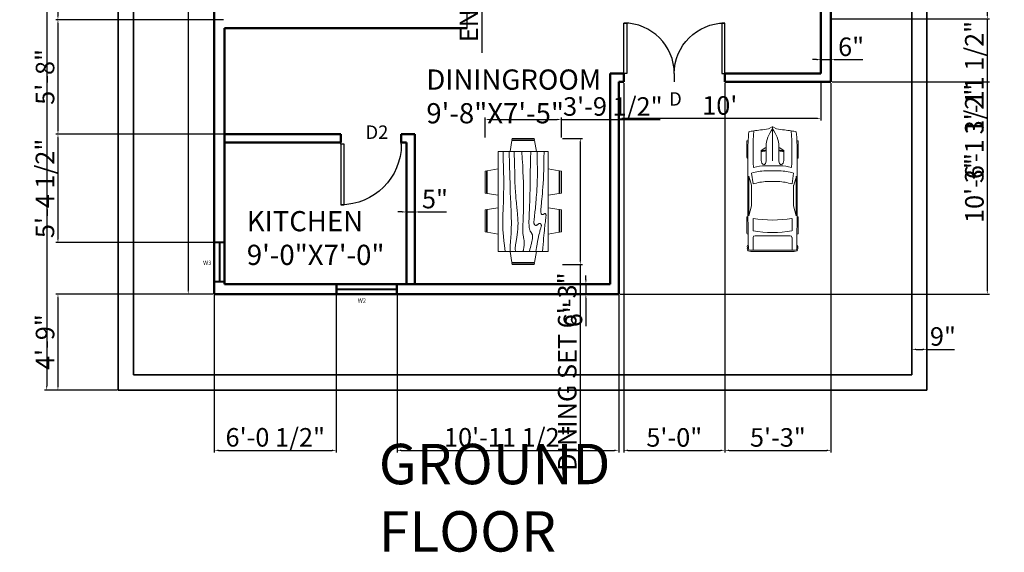
# Model space of a CAD drawing. Units: inches. Extents: x 2299 to 4423, y 1066 to 1805.
# Tile 1 of 7: x 2299 to 2884, y 1075 to 1391. Entities that reach past the tile are written whole.
import ezdxf

# ---------------------------------------------------------------- set-up
doc = ezdxf.new("R2010")
doc.units = ezdxf.units.IN
for name, color, linetype, lineweight in [('A-ANNO-DIMS', 2, 'Continuous', 18), ('A-ANNO-TEXT', 1, 'Continuous', 25), ('A-AREA-IDEN', 1, 'Continuous', 25), ('A-DOOR', 5, 'Continuous', 25), ('A-FLOR-STRS', 6, 'Continuous', 25), ('A-FURN', 8, 'Continuous', 18), ('A-GLAZ', 3, 'Continuous', 25), ('A-WALL', 7, 'Continuous', 50), ('C-PROP', 7, 'Continuous', 35)]:
    doc.layers.add(name, color=color, linetype=linetype, lineweight=lineweight)
doc.styles.get("Standard").update_dxf_attribs({"font": 'arial.ttf'})
doc.dimstyles.new('ISO-25', dxfattribs={"dimtxt": 11, "dimasz": 2.5, "dimexe": 1.25, "dimexo": 0.625, "dimtad": 1, "dimlunit": 4, "dimtxsty": 'Standard', "dimcen": 2.5, "dimadec": 0, "dimazin": 0, "dimtfac": 1, "dimtmove": 0, "dimatfit": 3, "dimfxl": 1, "dimarcsym": 0})

# ---------------------------------------------------------------- blocks, each defined once
blk = doc.blocks.new('*U2')
for p, q in [((0, 0), (0, -5)), ((30, 0), (30, -5))]:
    blk.add_line(p, q)
blk.add_lwpolyline([(0, 0), (0, 30), (1.75, 30), (1.75, 0)], close=True)
blk.add_arc((0, 0), 30, 0, 90)
blk = doc.blocks.new('Dining Set - 36 x 72 in.')
for p, q in [((-22.2343, 26.00059), (-23.4847, 17.99762)), ((-22.2304, 26), (-5.7608, 26)), ((-22, 27.5), (-22.1562, 26.50042)), ((-5.8416, 26.5), (-22.1534, 26.5)), ((-22, 27.5), (-6, 27.5)), ((-5.8437, 26.49966), (-6, 27.5)), ((-4.5152, 17.99762), (-5.7655, 25.99926)), ((5.7657, 26.00059), (4.5153, 17.99762)), ((5.7696, 26), (22.2392, 26)), ((6, 27.5), (5.8438, 26.50042)), ((22.1584, 26.5), (5.8466, 26.5)), ((6, 27.5), (22, 27.5)), ((22.1563, 26.49966), (22, 27.5)), ((23.4848, 17.99762), (22.2345, 25.99926)), ((36, 18), (-36, 18)), ((-36, 18), (-36, -18)), ((36, -18), (36, 18)), ((-45.5, 8), (-44.5004, 8.15617)), ((-45.5, 8), (-45.5, -8)), ((-44.5, -8.15843), (-44.5, 8.15338)), ((-44.0006, 8.23428), (-35.9976, 9.48474)), ((-44, 8.23041), (-44, -8.23915)), ((44.0006, 8.23428), (35.9976, 9.48474)), ((44, 8.23041), (44, -8.23915)), ((44.5, -8.15843), (44.5, 8.15338)), ((45.5, 8), (44.5005, 8.15617)), ((45.5, 8), (45.5, -8)), ((-44.4997, -8.15631), (-45.5, -8)), ((-35.9976, -9.48476), (-43.9993, -8.2345)), ((35.9976, -9.48476), (43.9993, -8.2345)), ((44.4997, -8.15631), (45.5, -8)), ((-36, -18), (36, -18)), ((-22.2343, -26.0006), (-23.4847, -17.99762)), ((-4.5152, -17.99762), (-5.7655, -25.99928)), ((5.7657, -26.0006), (4.5153, -17.99762)), ((23.4848, -17.99762), (22.2345, -25.99928)), ((-22.2304, -26), (-5.7608, -26)), ((-22, -27.5), (-22.1562, -26.50044)), ((-5.8416, -26.5), (-22.1534, -26.5)), ((-22, -27.5), (-6, -27.5)), ((-5.8437, -26.49967), (-6, -27.5)), ((5.7696, -26), (22.2392, -26)), ((6, -27.5), (5.8438, -26.50044)), ((22.1584, -26.5), (5.8466, -26.5)), ((6, -27.5), (22, -27.5)), ((22.1563, -26.49967), (22, -27.5))]:
    blk.add_line(p, q)
for points in [[(-36, 15), (-31.1772, 14.97754), (-26.8079, 14.91406), (-22.8538, 14.81543), (-19.276, 14.6875), (-16.0362, 14.53613), (-13.0957, 14.36718), (-10.4159, 14.18652), (-7.9583, 14), (-5.6904, 13.81315), (-3.6035, 13.63021), (-1.6954, 13.45508), (0.0365, 13.29166), (1.5945, 13.14388), (2.9811, 13.01562), (4.1988, 12.9108), (5.25, 12.83333), (6.1393, 12.78613), (6.8802, 12.76823), (7.4883, 12.77767), (7.9792, 12.8125), (8.3685, 12.87077), (8.6719, 12.95052), (8.9049, 13.0498), (9.0833, 13.16666), (9.2205, 13.29899), (9.3216, 13.44401), (9.3895, 13.59879), (9.4271, 13.76041), (9.4373, 13.92594), (9.4232, 14.09245), (9.3875, 14.257), (9.3333, 14.41666), (9.2638, 14.56917), (9.1836, 14.71484), (9.0975, 14.85465), (9.0104, 14.98958), (8.9272, 15.1206), (8.8529, 15.2487), (8.7922, 15.37483), (8.75, 15.5), (8.7305, 15.62467), (8.7344, 15.74739), (8.7617, 15.86621), (8.8125, 15.97916), (8.8867, 16.08431), (8.9844, 16.17968), (9.1055, 16.26334), (9.25, 16.33333), (9.4189, 16.38802), (9.6172, 16.42708), (9.8506, 16.45052), (10.125, 16.45833), (10.4463, 16.45052), (10.8203, 16.42708), (11.2529, 16.38802), (11.75, 16.33333), (12.3184, 16.26318), (12.9694, 16.17838), (13.7151, 16.07991), (14.5677, 15.96875), (15.5395, 15.84586), (16.6426, 15.71224), (17.8893, 15.56884), (19.2917, 15.41666), (20.859, 15.25667), (22.5879, 15.08984), (24.4721, 14.91715), (26.5052, 14.73958), (28.6809, 14.5581), (30.9929, 14.3737), (33.4347, 14.18733), (36, 14)], [(-36, 10), (-28.9766, 10.14274), (-23.1725, 10.20442), (-18.4241, 10.19775), (-14.5677, 10.13541), (-11.4399, 10.03011), (-8.877, 9.89453), (-6.7154, 9.74137), (-4.7917, 9.58333), (-2.9698, 9.43082), (-1.2246, 9.28515), (0.4415, 9.14534), (2.026, 9.01041), (3.5266, 8.87939), (4.9408, 8.7513), (6.266, 8.62516), (7.5, 8.5), (8.6411, 8.37549), (9.6914, 8.2539), (10.6538, 8.13818), (11.5312, 8.03125), (12.3267, 7.93603), (13.043, 7.85547), (13.6831, 7.79248), (14.25, 7.75), (14.7471, 7.7303), (15.1797, 7.73307), (15.5537, 7.75732), (15.875, 7.80208), (16.1494, 7.86637), (16.3828, 7.94922), (16.5811, 8.04964), (16.75, 8.16666), (16.8944, 8.29915), (17.0143, 8.44531), (17.1089, 8.60319), (17.1771, 8.77083), (17.218, 8.94629), (17.2305, 9.1276), (17.2137, 9.31282), (17.1667, 9.5), (17.0895, 9.6875), (16.987, 9.875), (16.8649, 10.0625), (16.7292, 10.25), (16.5856, 10.4375), (16.4401, 10.625), (16.2985, 10.8125), (16.1667, 11), (16.05, 11.18733), (15.9518, 11.3737), (15.8752, 11.5581), (15.8229, 11.73958), (15.798, 11.91715), (15.8034, 12.08984), (15.842, 12.25667), (15.9167, 12.41666), (16.0295, 12.56836), (16.1784, 12.70833), (16.3605, 12.83268), (16.5729, 12.9375), (16.8127, 13.01888), (17.0768, 13.07291), (17.3625, 13.0957), (17.6667, 13.08333), (17.9894, 13.03312), (18.3418, 12.94726), (18.7382, 12.82918), (19.1927, 12.68229), (19.7195, 12.51001), (20.3327, 12.31575), (21.0465, 12.10294), (21.875, 11.875), (22.8357, 11.63354), (23.959, 11.37304), (25.2786, 11.08618), (26.8282, 10.76562), (28.6414, 10.40405), (30.752, 9.99414), (33.1936, 9.52856), (36, 9)], [(-36, 5.5), (-30.7157, 5.3348), (-26.069, 5.20963), (-21.9946, 5.11767), (-18.4271, 5.05208), (-15.3009, 5.00602), (-12.5508, 4.97265), (-10.1112, 4.94515), (-7.9167, 4.91666), (-5.909, 4.88167), (-4.0586, 4.83984), (-2.3429, 4.79215), (-0.7396, 4.73958), (0.7739, 4.6831), (2.22, 4.6237), (3.6213, 4.56233), (5, 4.5), (6.373, 4.43782), (7.7344, 4.3776), (9.0723, 4.32129), (10.375, 4.27083), (11.6309, 4.22819), (12.8281, 4.19531), (13.9551, 4.17415), (15, 4.16666), (15.954, 4.17448), (16.819, 4.19791), (17.6001, 4.23698), (18.3021, 4.29166), (18.9299, 4.36198), (19.4883, 4.44791), (19.9823, 4.54948), (20.4167, 4.66666), (20.7969, 4.79899), (21.1302, 4.94401), (21.4245, 5.09879), (21.6875, 5.26041), (21.9271, 5.42594), (22.1511, 5.59245), (22.3672, 5.757), (22.5834, 5.91666), (22.8065, 6.06868), (23.0404, 6.21093), (23.2879, 6.34147), (23.5521, 6.45833), (23.8358, 6.55957), (24.142, 6.64323), (24.4735, 6.70735), (24.8334, 6.75), (25.2235, 6.76969), (25.642, 6.76692), (26.0858, 6.74267), (26.5521, 6.69791), (27.0379, 6.63362), (27.5404, 6.55078), (28.0565, 6.45036), (28.5834, 6.33333), (29.1242, 6.19987), (29.7071, 6.04687), (30.3661, 5.87044), (31.1354, 5.66666), (32.0493, 5.43164), (33.142, 5.16146), (34.4475, 4.85221), (36, 4.5)], [(-36, -1), (-30.7915, -0.6591), (-26.0195, -0.38216), (-21.6519, -0.16284), (-17.6563, 0.00521), (-14.0005, 0.12833), (-10.6523, 0.21289), (-7.5796, 0.26522), (-4.75, 0.29166), (-2.134, 0.29793), (0.2878, 0.28711), (2.5317, 0.26163), (4.6146, 0.22396), (6.5529, 0.17651), (8.3633, 0.12174), (10.0623, 0.06209), (11.6667, 0), (13.1899, -0.06201), (14.6341, -0.1211), (15.9982, -0.17432), (17.2813, -0.21875), (18.4823, -0.25147), (19.6003, -0.26953), (20.6343, -0.27002), (21.5834, -0.25), (22.4481, -0.20768), (23.2357, -0.14584), (23.9549, -0.06836), (24.6146, 0.02083), (25.2235, 0.11784), (25.7904, 0.21875), (26.3241, 0.31966), (26.8334, 0.41666), (27.3265, 0.50618), (27.8099, 0.58593), (28.2894, 0.65397), (28.7709, 0.70833), (29.2601, 0.74707), (29.763, 0.76823), (30.2855, 0.76985), (30.8334, 0.75), (31.4088, 0.70784), (31.9994, 0.64713), (32.589, 0.57275), (33.1615, 0.48958), (33.7008, 0.4025), (34.1908, 0.3164), (34.6153, 0.23616), (34.9584, 0.16666), (35.2099, 0.11165), (35.3848, 0.07031), (35.504, 0.04069), (35.5886, 0.02083), (35.6594, 0.00879), (35.7377, 0.0026), (35.8442, 0.00032), (36, 0)], [(-36, -6.5), (-27.1843, -6.31267), (-20.084, -6.1263), (-14.469, -5.9419), (-10.1094, -5.76042), (-6.7752, -5.58285), (-4.2363, -5.41016), (-2.2629, -5.24333), (-0.625, -5.08334), (0.8708, -4.93099), (2.2715, -4.78646), (3.5872, -4.64974), (4.8281, -4.52084), (6.0046, -4.39974), (7.127, -4.28646), (8.2053, -4.18099), (9.25, -4.08334), (10.2705, -3.99382), (11.2734, -3.91407), (12.2647, -3.84603), (13.25, -3.79167), (14.2354, -3.75293), (15.2266, -3.73177), (16.2295, -3.73015), (17.25, -3.75), (18.2912, -3.79248), (19.3451, -3.85547), (20.4009, -3.93604), (21.4479, -4.03125), (22.4754, -4.13819), (23.4727, -4.25391), (24.4289, -4.37549), (25.3334, -4.5), (26.1785, -4.62492), (26.9694, -4.74935), (27.7145, -4.87281), (28.4219, -4.99479), (29.1, -5.11483), (29.7572, -5.23242), (30.4016, -5.34709), (31.0417, -5.45834), (31.6837, -5.56437), (32.3262, -5.65821), (32.9658, -5.73153), (33.599, -5.77604), (34.2224, -5.78345), (34.8327, -5.74545), (35.4264, -5.65373), (36, -5.5)], [(-36, -10), (-26.4022, -9.81299), (-18.4675, -9.62891), (-11.9839, -9.45069), (-6.7396, -9.28125), (-2.5226, -9.12354), (0.8789, -8.98047), (3.6769, -8.85498), (6.0833, -8.75), (8.2767, -8.66765), (10.3021, -8.60677), (12.1712, -8.56543), (13.8958, -8.54167), (15.4876, -8.53353), (16.9583, -8.53907), (18.3197, -8.55632), (19.5834, -8.58334), (20.7616, -8.61841), (21.8685, -8.66081), (22.9188, -8.71004), (23.9271, -8.76563), (24.9081, -8.82707), (25.8763, -8.89388), (26.8465, -8.96558), (27.8334, -9.04167), (28.8474, -9.12118), (29.8828, -9.20117), (30.93, -9.27824), (31.9792, -9.34896), (33.0205, -9.40991), (34.0443, -9.45768), (35.0407, -9.48885), (36, -9.5)], [(-36, -14.5), (-30.0881, -14.33513), (-25.0332, -14.21224), (-20.7312, -14.12647), (-17.0781, -14.07292), (-13.97, -14.04671), (-11.3027, -14.04297), (-8.9724, -14.05681), (-6.875, -14.08334), (-4.9224, -14.11833), (-3.0905, -14.16016), (-1.3709, -14.20785), (0.2448, -14.26042), (1.7647, -14.3169), (3.1973, -14.3763), (4.5507, -14.43767), (5.8333, -14.5), (7.0554, -14.5621), (8.235, -14.62175), (9.3922, -14.67652), (10.5469, -14.72396), (11.7192, -14.76164), (12.929, -14.78711), (14.1965, -14.79794), (15.5417, -14.79167), (16.9933, -14.76424), (18.6152, -14.70508), (20.4804, -14.60197), (22.6615, -14.44271), (25.2312, -14.21509), (28.2624, -13.9069), (31.8277, -13.50594), (36, -13)]]:
    blk.add_lwpolyline(points)
blk = doc.blocks.new('*U11')
for p, q in [((21.1, 37.4), (21.1, 36.8)), ((46.6, 38.9), (22.4, 38.9)), ((47.8, 37.4), (47.8, 37.4)), ((70, 31.5), (86.4, 29.4)), ((88, 31.9), (74.8, 35.9)), ((134.3, 35.6), (119.3, 31.8)), ((135.5, 37.1), (135.5, 37.4)), ((136.7, 38.9), (160.9, 38.9)), ((162.1, 37.4), (162.1, 36.8)), ((186.5, -33.5), (186.5, 33.5)), ((188.4, -32.8), (188.4, 32.8)), ((32.3, 11.6), (36.1, 17.2)), ((36.1, 17.2), (50.9, 17.2)), ((138.4, 29.4), (157.2, 29.4)), ((164.5, 26.4), (164.5, -26.4)), ((186.5, 29.4), (167, 29.4)), ((3.3, 6.1), (0.1, 0.4)), ((29.8, 9.5), (51.7, 9.5)), ((32.1, 9.5), (32.1, 11.2)), ((58.9, -10.8), (58.9, 10.8)), ((66.6, -10.5), (66.6, 10.5)), ((82.7, 8.5), (82.7, -8.5)), ((186.5, -10.5), (186.5, 10.5)), ((0, 0), (51.7, 0)), ((0.1, -0.4), (3.3, -6.1)), ((29.8, -9.5), (51.7, -9.5)), ((32.1, -9.5), (32.1, -11.2)), ((32.3, -11.6), (36.1, -17.2)), ((36.1, -17.2), (50.9, -17.2)), ((86.4, -29.4), (70, -31.5)), ((157.2, -29.4), (138.4, -29.4)), ((167, -29.4), (186.5, -29.4)), ((21.1, -37.4), (21.1, -36.8)), ((46.6, -38.9), (22.4, -38.9)), ((47.8, -37.4), (47.8, -37.4)), ((88, -31.9), (74.8, -35.9)), ((134.3, -35.6), (119.3, -31.8)), ((135.5, -37.1), (135.5, -37.4)), ((136.7, -38.9), (160.9, -38.9)), ((162.1, -37.4), (162.1, -36.8))]:
    blk.add_line(p, q)
for centre, major_axis, ratio, start_param, end_param in [((266, -27.5), (0, 313.3), 0.842304, 1.367076, 1.39176), ((37.5, -594), (0, -623.3), 0.842304, 3.096046, 3.200911), ((41.2, -490.9), (0, 528.2), 0.842304, 0.00281, 0.075598), ((22.4, 37.4), (0, -1.48), 0.842304, 3.141593, 4.712389), ((64.5, -10555.6), (0, 10593), 0.842304, -0.013397, 0.002797), ((46.6, 37.4), (0, 1.48), 0.842304, -1.570796, 0), ((135.3, 5.4), (0, 81.8), 0.842304, 1.245306, 1.50788), ((64.5, -10555.6), (0, -10591.5), 0.842304, 3.133765, 3.140441), ((95.8, -3666.4), (0, -3698.2), 0.842304, 3.134049, 3.144098), ((136.7, 37.4), (0, -1.48), 0.842304, 3.141593, 4.712389), ((160.9, 37.4), (0, 1.48), 0.842304, -1.570796, 0), ((180.6, 35.8), (0, 2.22), 0.842304, -0.013017, 1.249894), ((64.5, -10556.4), (0, 10595.3), 0.842304, -0.013397, -0.013017), ((184, 32.8), (0, -5.25), 0.842304, 1.570796, 3.128196), ((184, 33.5), (0, -2.96), 0.842304, 1.570796, 3.128196), ((-204.5, 52.4), (0, -251), 0.842304, 1.385369, 1.434372), ((259.2, -27.5), (0, -305.3), 0.842304, 4.528606, 4.561838), ((13, 17), (0, 27.4), 0.842304, 4.435146, 4.718221), ((14.2, 17), (0, 27.4), 0.842304, 4.435146, 4.718221), ((50.8, 13.3), (6.34, -0.36), 0.603834, -1.395552, 1.581315), ((134.4, 5.4), (0, -89.8), 0.842304, 4.449482, 4.652344), ((149.6, 2.8), (0, -79.6), 0.842304, 4.372215, 4.640744), ((17.1, 0), (0, 147), 0.842304, 4.511394, 4.913384), ((35.9, 0), (0, 147), 0.842304, 4.511394, 4.913384), ((167, 26.4), (0, 2.96), 0.842304, 0, 1.570796), ((0.6, 0), (0, -0.74), 0.842304, 4.131459, 5.293319), ((29.8, -46.7), (0, 56.2), 0.842304, 0, 0.590319), ((32.7, 11.2), (0, 0.74), 0.842304, 0.879714, 1.570796), ((-204.5, -52.4), (0, 251), 0.842304, -1.434372, -1.385369), ((29.8, 46.7), (0, 56.2), 0.842304, 2.551274, 3.141593), ((32.7, -11.2), (0, -0.74), 0.842304, 4.712389, 5.403472), ((13, -17), (0, -27.4), 0.842304, 1.564964, 1.848039), ((14.2, -17), (0, -27.4), 0.842304, 1.564964, 1.848039), ((134.4, -5.4), (0, -89.8), 0.842304, -1.510751, -1.307889), ((135.3, -5.4), (0, -81.8), 0.842304, -1.50788, -1.245306), ((149.6, -2.8), (0, -79.6), 0.842304, -1.499151, -1.230623), ((259.2, 27.5), (0, 305.3), 0.842304, 1.721348, 1.754579), ((266, 27.5), (0, 313.3), 0.842304, 1.749832, 1.774517), ((37.5, 594), (0, -623.3), 0.842304, -0.059319, 0.045547), ((167, -26.4), (0, -2.96), 0.842304, 4.712389, 6.283185), ((41.2, 490.9), (0, -528.2), 0.842304, -0.075598, -0.00281), ((22.4, -37.4), (0, 1.48), 0.842304, 1.570796, 3.141593), ((64.5, 10555.6), (0, 10593), 0.842304, 3.138796, 3.15499), ((46.6, -37.4), (0, -1.48), 0.842304, 0, 1.570796), ((64.5, 10555.6), (0, -10591.5), 0.842304, 0.001152, 0.007828), ((95.8, 3666.4), (0, -3698.2), 0.842304, -0.002505, 0.007544), ((136.7, -37.4), (0, -1.48), 0.842304, -1.570796, 0), ((160.9, -37.4), (0, 1.48), 0.842304, 3.141593, 4.712389), ((180.6, -35.8), (0, -2.22), 0.842304, -1.249894, 0.013017), ((64.5, 10556.4), (0, 10595.3), 0.842304, 3.15461, 3.15499), ((184, -32.8), (0, -5.25), 0.842304, 0.013397, 1.570796), ((184, -33.5), (0, 2.96), 0.842304, 3.15499, 4.712389)]:
    blk.add_ellipse(centre, major_axis=major_axis, ratio=ratio, start_param=start_param, end_param=end_param)
at = {"extrusion": (0, 0, -1)}
blk.add_ellipse((50.8, -13.3), major_axis=(6.34, 0.36), ratio=0.603834, start_param=-1.395552, end_param=1.581315, dxfattribs=at)
blk = doc.blocks.new('*D12')
at = {"layer": 'A-ANNO-DIMS', "color": 0, "lineweight": -2, "transparency": 16777216}
for p, q in [((2654.83, 1353.32), (2654.83, 1331.09)), ((2774.83, 1353.32), (2774.83, 1331.09)), ((2772.33, 1332.34), (2657.33, 1332.34))]:
    blk.add_line(p, q, dxfattribs=at)
at = {"layer": 'A-ANNO-DIMS', "color": 0, "transparency": 16777216}
for points in [[(2657.33, 1332.76), (2657.33, 1331.92), (2654.83, 1332.34)], [(2772.33, 1332.76), (2772.33, 1331.92), (2774.83, 1332.34)]]:
    blk.add_solid(points, dxfattribs=at)
at = {"layer": 'Defpoints', "color": 0, "transparency": 16777216}
for p in [(2654.83, 1353.95), (2774.83, 1353.95), (2654.83, 1332.34)]:
    blk.add_point(p, dxfattribs=at)
at = {"layer": 'A-ANNO-DIMS', "color": 0, "transparency": 16777216, "insert": (2714.83, 1338.58), "char_height": 11, "attachment_point": 5}
blk.add_mtext("10'", dxfattribs=at)
blk = doc.blocks.new('*D13')
at = {"layer": 'A-ANNO-DIMS', "color": 0, "lineweight": -2, "transparency": 16777216}
for p, q in [((2635.37, 1236.45), (2635.37, 1238.95)), ((2636.27, 1233.95), (2634.12, 1233.95)), ((2635.37, 1233.95), (2635.37, 1227.95)), ((2636.27, 1227.95), (2634.12, 1227.95)), ((2635.37, 1225.45), (2635.37, 1208.99))]:
    blk.add_line(p, q, dxfattribs=at)
at = {"layer": 'A-ANNO-DIMS', "color": 0, "transparency": 16777216}
for points in [[(2634.95, 1236.45), (2635.78, 1236.45), (2635.37, 1233.95)], [(2634.95, 1225.45), (2635.78, 1225.45), (2635.37, 1227.95)]]:
    blk.add_solid(points, dxfattribs=at)
at = {"layer": 'Defpoints', "color": 0, "transparency": 16777216}
for p in [(2636.89, 1233.95), (2635.37, 1227.95), (2636.89, 1227.95)]:
    blk.add_point(p, dxfattribs=at)
at = {"layer": 'A-ANNO-DIMS', "color": 0, "transparency": 16777216, "insert": (2629.13, 1215.97), "char_height": 11, "attachment_point": 5, "rotation": 90}
blk.add_mtext('6"', dxfattribs=at)
blk = doc.blocks.new('*D14')
at = {"layer": 'A-ANNO-DIMS', "color": 0, "lineweight": -2, "transparency": 16777216}
for p, q in [((2828.83, 1180.57), (2828.83, 1196.38)), ((2831.33, 1195.13), (2835.33, 1195.13)), ((2837.83, 1180.57), (2837.83, 1196.38)), ((2837.83, 1195.13), (2854.23, 1195.13))]:
    blk.add_line(p, q, dxfattribs=at)
at = {"layer": 'A-ANNO-DIMS', "color": 0, "transparency": 16777216}
for points in [[(2831.33, 1195.55), (2831.33, 1194.71), (2828.83, 1195.13)], [(2835.33, 1195.55), (2835.33, 1194.71), (2837.83, 1195.13)]]:
    blk.add_solid(points, dxfattribs=at)
at = {"layer": 'Defpoints', "color": 0, "transparency": 16777216}
for p in [(2837.83, 1195.13), (2828.83, 1179.95), (2837.83, 1179.95)]:
    blk.add_point(p, dxfattribs=at)
at = {"layer": 'A-ANNO-DIMS', "color": 0, "transparency": 16777216, "insert": (2847.28, 1201.37), "char_height": 11, "attachment_point": 5}
blk.add_mtext('9"', dxfattribs=at)
blk = doc.blocks.new('*D15')
at = {"layer": 'A-ANNO-DIMS', "color": 0, "lineweight": -2, "transparency": 16777216}
for p, q in [((2526.33, 1276.74), (2523.83, 1276.74)), ((2528.83, 1276.57), (2528.83, 1277.99)), ((2528.83, 1276.74), (2533.83, 1276.74)), ((2533.83, 1276.57), (2533.83, 1277.99)), ((2536.33, 1276.74), (2552.73, 1276.74))]:
    blk.add_line(p, q, dxfattribs=at)
at = {"layer": 'A-ANNO-DIMS', "color": 0, "transparency": 16777216}
for points in [[(2526.33, 1277.15), (2526.33, 1276.32), (2528.83, 1276.74)], [(2536.33, 1277.15), (2536.33, 1276.32), (2533.83, 1276.74)]]:
    blk.add_solid(points, dxfattribs=at)
at = {"layer": 'Defpoints', "color": 0, "transparency": 16777216}
for p in [(2528.83, 1275.95), (2533.83, 1276.74), (2533.83, 1275.95)]:
    blk.add_point(p, dxfattribs=at)
at = {"layer": 'A-ANNO-DIMS', "color": 0, "transparency": 16777216, "insert": (2545.78, 1282.96), "char_height": 11, "attachment_point": 5}
blk.add_mtext('5"', dxfattribs=at)
blk = doc.blocks.new('*D21')
at = {"layer": 'A-ANNO-DIMS', "color": 0, "lineweight": -2, "transparency": 16777216}
for p, q in [((2357.21, 1746.95), (2314.11, 1746.95)), ((2315.36, 1744.45), (2315.36, 1173.45)), ((2357.21, 1170.95), (2314.11, 1170.95))]:
    blk.add_line(p, q, dxfattribs=at)
at = {"layer": 'A-ANNO-DIMS', "color": 0, "transparency": 16777216}
for points in [[(2314.94, 1744.45), (2315.77, 1744.45), (2315.36, 1746.95)], [(2314.94, 1173.45), (2315.77, 1173.45), (2315.36, 1170.95)]]:
    blk.add_solid(points, dxfattribs=at)
at = {"layer": 'Defpoints', "color": 0, "transparency": 16777216}
for p in [(2357.83, 1746.95), (2315.36, 1170.95), (2357.83, 1170.95)]:
    blk.add_point(p, dxfattribs=at)
at = {"layer": 'A-ANNO-DIMS', "color": 0, "transparency": 16777216, "insert": (2309.11, 1458.95), "char_height": 11, "attachment_point": 5, "rotation": 90}
blk.add_mtext("48'", dxfattribs=at)
blk = doc.blocks.new('*D23')
at = {"layer": 'A-ANNO-DIMS', "color": 0, "lineweight": -2, "transparency": 16777216}
for p, q in [((2414.21, 1689.95), (2398.11, 1689.95)), ((2399.36, 1687.45), (2399.36, 1230.45)), ((2414.21, 1227.95), (2398.11, 1227.95))]:
    blk.add_line(p, q, dxfattribs=at)
at = {"layer": 'A-ANNO-DIMS', "color": 0, "transparency": 16777216}
for points in [[(2398.94, 1687.45), (2399.78, 1687.45), (2399.36, 1689.95)], [(2398.94, 1230.45), (2399.78, 1230.45), (2399.36, 1227.95)]]:
    blk.add_solid(points, dxfattribs=at)
at = {"layer": 'Defpoints', "color": 0, "transparency": 16777216}
for p in [(2414.83, 1689.95), (2399.36, 1227.95), (2414.83, 1227.95)]:
    blk.add_point(p, dxfattribs=at)
at = {"layer": 'A-ANNO-DIMS', "color": 0, "transparency": 16777216, "insert": (2393.12, 1458.95), "char_height": 11, "attachment_point": 5, "rotation": 90}
blk.add_mtext('38\'-6"', dxfattribs=at)
blk = doc.blocks.new('*D30')
at = {"layer": 'A-ANNO-DIMS', "color": 0, "lineweight": -2, "transparency": 16777216}
for p, q in [((2774.83, 1359.57), (2774.83, 1368.45)), ((2780.83, 1359.57), (2780.83, 1368.45)), ((2772.33, 1367.2), (2769.83, 1367.2)), ((2774.83, 1367.2), (2780.83, 1367.2)), ((2783.33, 1367.2), (2799.79, 1367.2))]:
    blk.add_line(p, q, dxfattribs=at)
at = {"layer": 'A-ANNO-DIMS', "color": 0, "transparency": 16777216}
for points in [[(2772.33, 1367.62), (2772.33, 1366.78), (2774.83, 1367.2)], [(2783.33, 1367.62), (2783.33, 1366.78), (2780.83, 1367.2)]]:
    blk.add_solid(points, dxfattribs=at)
at = {"layer": 'Defpoints', "color": 0, "transparency": 16777216}
for p in [(2780.83, 1367.2), (2774.83, 1358.95), (2780.83, 1358.95)]:
    blk.add_point(p, dxfattribs=at)
at = {"layer": 'A-ANNO-DIMS', "color": 0, "transparency": 16777216, "insert": (2792.81, 1373.44), "char_height": 11, "attachment_point": 5}
blk.add_mtext('6"', dxfattribs=at)
blk = doc.blocks.new('WIN-600')
for p, q in [((0, 6), (24.07, 6)), ((0, 0), (0, 6)), ((0.5, 0), (0.5, 6)), ((23.57, 6), (23.57, 0)), ((24.07, 6), (24.07, 0)), ((24.07, 0), (0, 0)), ((0.5, 3.2), (23.57, 3.2)), ((0.5, 2.8), (23.57, 2.8))]:
    blk.add_line(p, q)
blk = doc.blocks.new('WIN-900')
for p, q in [((0, 6), (36.07, 6)), ((0, 0), (0, 6)), ((0.5, 0), (0.5, 6)), ((35.57, 6), (35.57, 0)), ((36.07, 6), (36.07, 0)), ((36.07, 0), (0, 0)), ((0.5, 3.2), (35.57, 3.2)), ((0.5, 2.8), (35.57, 2.8))]:
    blk.add_line(p, q)
blk = doc.blocks.new('*D40')
at = {"layer": 'A-ANNO-DIMS', "color": 0, "lineweight": -2, "transparency": 16777216}
for p, q in [((2566.71, 1666.57), (2574.84, 1666.57)), ((2573.59, 1664.07), (2573.59, 1619.02)), ((2566.71, 1616.52), (2574.84, 1616.52)), ((2573.59, 1616.52), (2573.59, 1371.29))]:
    blk.add_line(p, q, dxfattribs=at)
at = {"layer": 'A-ANNO-DIMS', "color": 0, "transparency": 16777216}
for points in [[(2573.18, 1664.07), (2574.01, 1664.07), (2573.59, 1666.57)], [(2573.18, 1619.02), (2574.01, 1619.02), (2573.59, 1616.52)]]:
    blk.add_solid(points, dxfattribs=at)
at = {"layer": 'Defpoints', "color": 0, "transparency": 16777216}
for p in [(2566.08, 1666.57), (2566.08, 1616.52), (2573.59, 1616.52)]:
    blk.add_point(p, dxfattribs=at)
at = {"layer": 'A-ANNO-DIMS', "color": 0, "transparency": 16777216, "insert": (2567.35, 1492.65), "char_height": 11, "attachment_point": 5, "rotation": 90}
blk.add_mtext('ENTERTAINMENT UNIT 4\'-2" TYP.', dxfattribs=at)
blk = doc.blocks.new('*D56')
at = {"layer": 'A-ANNO-DIMS', "color": 0, "lineweight": -2, "transparency": 16777216}
for p, q in [((2621.43, 1320.41), (2633.29, 1320.41)), ((2632.04, 1317.91), (2632.04, 1247.99)), ((2621.43, 1245.49), (2633.29, 1245.49)), ((2632.04, 1245.49), (2632.04, 1120.84))]:
    blk.add_line(p, q, dxfattribs=at)
at = {"layer": 'A-ANNO-DIMS', "color": 0, "transparency": 16777216}
for points in [[(2631.63, 1317.91), (2632.46, 1317.91), (2632.04, 1320.41)], [(2631.63, 1247.99), (2632.46, 1247.99), (2632.04, 1245.49)]]:
    blk.add_solid(points, dxfattribs=at)
at = {"layer": 'Defpoints', "color": 0, "transparency": 16777216}
for p in [(2620.81, 1320.41), (2620.81, 1245.49), (2632.04, 1245.49)]:
    blk.add_point(p, dxfattribs=at)
at = {"layer": 'A-ANNO-DIMS', "color": 0, "transparency": 16777216, "insert": (2625.73, 1181.91), "char_height": 11, "attachment_point": 5, "rotation": 90}
blk.add_mtext('DINING SET 6\'-3"', dxfattribs=at)
blk = doc.blocks.new('*D57')
at = {"layer": 'A-ANNO-DIMS', "color": 0, "lineweight": -2, "transparency": 16777216}
for p, q in [((2575.53, 1321.03), (2575.53, 1332.89)), ((2620.81, 1321.03), (2620.81, 1332.89)), ((2578.03, 1331.64), (2618.31, 1331.64)), ((2620.81, 1331.64), (2679.42, 1331.64))]:
    blk.add_line(p, q, dxfattribs=at)
at = {"layer": 'A-ANNO-DIMS', "color": 0, "transparency": 16777216}
for points in [[(2578.03, 1332.06), (2578.03, 1331.23), (2575.53, 1331.64)], [(2618.31, 1332.06), (2618.31, 1331.23), (2620.81, 1331.64)]]:
    blk.add_solid(points, dxfattribs=at)
at = {"layer": 'Defpoints', "color": 0, "transparency": 16777216}
for p in [(2620.81, 1331.64), (2575.53, 1320.41), (2620.81, 1320.41)]:
    blk.add_point(p, dxfattribs=at)
at = {"layer": 'A-ANNO-DIMS', "color": 0, "transparency": 16777216, "insert": (2651.36, 1337.96), "char_height": 11, "attachment_point": 5}
blk.add_mtext('3\'-9 1/2"', dxfattribs=at)
blk = doc.blocks.new('*D73')
at = {"layer": 'A-ANNO-DIMS', "color": 0, "lineweight": -2, "transparency": 16777216}
for p, q in [((2420.21, 1539.95), (2320.78, 1539.95)), ((2322.03, 1537.45), (2322.03, 1393.45)), ((2420.21, 1390.95), (2320.78, 1390.95))]:
    blk.add_line(p, q, dxfattribs=at)
at = {"layer": 'A-ANNO-DIMS', "color": 0, "transparency": 16777216}
for points in [[(2321.62, 1537.45), (2322.45, 1537.45), (2322.03, 1539.95)], [(2321.62, 1393.45), (2322.45, 1393.45), (2322.03, 1390.95)]]:
    blk.add_solid(points, dxfattribs=at)
at = {"layer": 'Defpoints', "color": 0, "transparency": 16777216}
for p in [(2420.83, 1539.95), (2322.03, 1390.95), (2420.83, 1390.95)]:
    blk.add_point(p, dxfattribs=at)
at = {"layer": 'A-ANNO-DIMS', "color": 0, "transparency": 16777216, "insert": (2315.79, 1465.45), "char_height": 11, "attachment_point": 5, "rotation": 90}
blk.add_mtext('12\'-5"', dxfattribs=at)
blk = doc.blocks.new('*D74')
at = {"layer": 'A-ANNO-DIMS', "color": 0, "lineweight": -2, "transparency": 16777216}
for p, q in [((2420.21, 1390.95), (2320.78, 1390.95)), ((2322.03, 1388.45), (2322.03, 1325.45)), ((2420.21, 1322.95), (2320.78, 1322.95))]:
    blk.add_line(p, q, dxfattribs=at)
at = {"layer": 'A-ANNO-DIMS', "color": 0, "transparency": 16777216}
for points in [[(2321.62, 1388.45), (2322.45, 1388.45), (2322.03, 1390.95)], [(2321.62, 1325.45), (2322.45, 1325.45), (2322.03, 1322.95)]]:
    blk.add_solid(points, dxfattribs=at)
at = {"layer": 'Defpoints', "color": 0, "transparency": 16777216}
for p in [(2420.83, 1390.95), (2322.03, 1322.95), (2420.83, 1322.95)]:
    blk.add_point(p, dxfattribs=at)
at = {"layer": 'A-ANNO-DIMS', "color": 0, "transparency": 16777216, "insert": (2315.79, 1356.95), "char_height": 11, "attachment_point": 5, "rotation": 90}
blk.add_mtext('5\'-8"', dxfattribs=at)
blk = doc.blocks.new('*D75')
at = {"layer": 'A-ANNO-DIMS', "color": 0, "lineweight": -2, "transparency": 16777216}
for p, q in [((2420.21, 1322.95), (2320.78, 1322.95)), ((2322.03, 1320.45), (2322.03, 1261.02)), ((2414.21, 1258.52), (2320.78, 1258.52))]:
    blk.add_line(p, q, dxfattribs=at)
at = {"layer": 'A-ANNO-DIMS', "color": 0, "transparency": 16777216}
for points in [[(2321.62, 1320.45), (2322.45, 1320.45), (2322.03, 1322.95)], [(2321.62, 1261.02), (2322.45, 1261.02), (2322.03, 1258.52)]]:
    blk.add_solid(points, dxfattribs=at)
at = {"layer": 'Defpoints', "color": 0, "transparency": 16777216}
for p in [(2420.83, 1322.95), (2322.03, 1258.52), (2414.83, 1258.52)]:
    blk.add_point(p, dxfattribs=at)
at = {"layer": 'A-ANNO-DIMS', "color": 0, "transparency": 16777216, "insert": (2315.72, 1290.73), "char_height": 11, "attachment_point": 5, "rotation": 90}
blk.add_mtext('5\'-4 1/2"', dxfattribs=at)
blk = doc.blocks.new('*D76')
at = {"layer": 'A-ANNO-DIMS', "color": 0, "lineweight": -2, "transparency": 16777216}
for p, q in [((2414.21, 1227.95), (2320.78, 1227.95)), ((2322.03, 1225.45), (2322.03, 1173.45)), ((2357.21, 1170.95), (2320.78, 1170.95))]:
    blk.add_line(p, q, dxfattribs=at)
at = {"layer": 'A-ANNO-DIMS', "color": 0, "transparency": 16777216}
for points in [[(2321.62, 1225.45), (2322.45, 1225.45), (2322.03, 1227.95)], [(2321.62, 1173.45), (2322.45, 1173.45), (2322.03, 1170.95)]]:
    blk.add_solid(points, dxfattribs=at)
at = {"layer": 'Defpoints', "color": 0, "transparency": 16777216}
for p in [(2414.83, 1227.95), (2322.03, 1170.95), (2357.83, 1170.95)]:
    blk.add_point(p, dxfattribs=at)
at = {"layer": 'A-ANNO-DIMS', "color": 0, "transparency": 16777216, "insert": (2315.79, 1199.45), "char_height": 11, "attachment_point": 5, "rotation": 90}
blk.add_mtext('4\'-9"', dxfattribs=at)
blk = doc.blocks.new('*D81')
at = {"layer": 'A-ANNO-DIMS', "color": 0, "lineweight": -2, "transparency": 16777216}
for p, q in [((2781.46, 1438.95), (2874.88, 1438.95)), ((2873.63, 1436.45), (2873.63, 1393.85)), ((2781.46, 1391.35), (2874.88, 1391.35)), ((2873.63, 1391.35), (2873.63, 1324.19))]:
    blk.add_line(p, q, dxfattribs=at)
at = {"layer": 'A-ANNO-DIMS', "color": 0, "transparency": 16777216}
for points in [[(2873.22, 1436.45), (2874.05, 1436.45), (2873.63, 1438.95)], [(2873.22, 1393.85), (2874.05, 1393.85), (2873.63, 1391.35)]]:
    blk.add_solid(points, dxfattribs=at)
at = {"layer": 'Defpoints', "color": 0, "transparency": 16777216}
for p in [(2780.83, 1438.95), (2780.83, 1391.35), (2873.63, 1391.35)]:
    blk.add_point(p, dxfattribs=at)
at = {"layer": 'A-ANNO-DIMS', "color": 0, "transparency": 16777216, "insert": (2867.32, 1356.52), "char_height": 11, "attachment_point": 5, "rotation": 90}
blk.add_mtext('3\'-11 1/2"', dxfattribs=at)
blk = doc.blocks.new('*D82')
at = {"layer": 'A-ANNO-DIMS', "color": 0, "lineweight": -2, "transparency": 16777216}
for p, q in [((2781.46, 1391.35), (2874.88, 1391.35)), ((2873.63, 1388.85), (2873.63, 1356.45)), ((2781.46, 1353.95), (2874.88, 1353.95)), ((2873.63, 1353.95), (2873.63, 1295.33))]:
    blk.add_line(p, q, dxfattribs=at)
at = {"layer": 'A-ANNO-DIMS', "color": 0, "transparency": 16777216}
for points in [[(2873.22, 1388.85), (2874.05, 1388.85), (2873.63, 1391.35)], [(2873.22, 1356.45), (2874.05, 1356.45), (2873.63, 1353.95)]]:
    blk.add_solid(points, dxfattribs=at)
at = {"layer": 'Defpoints', "color": 0, "transparency": 16777216}
for p in [(2780.83, 1391.35), (2780.83, 1353.95), (2873.63, 1353.95)]:
    blk.add_point(p, dxfattribs=at)
at = {"layer": 'A-ANNO-DIMS', "color": 0, "transparency": 16777216, "insert": (2867.32, 1323.39), "char_height": 11, "attachment_point": 5, "rotation": 90}
blk.add_mtext('3\'-1 1/2"', dxfattribs=at)
blk = doc.blocks.new('*D83')
at = {"layer": 'A-ANNO-DIMS', "color": 0, "lineweight": -2, "transparency": 16777216}
for p, q in [((2781.46, 1353.95), (2874.88, 1353.95)), ((2873.63, 1351.45), (2873.63, 1230.45)), ((2655.46, 1227.95), (2874.88, 1227.95))]:
    blk.add_line(p, q, dxfattribs=at)
at = {"layer": 'A-ANNO-DIMS', "color": 0, "transparency": 16777216}
for points in [[(2873.22, 1351.45), (2874.05, 1351.45), (2873.63, 1353.95)], [(2873.22, 1230.45), (2874.05, 1230.45), (2873.63, 1227.95)]]:
    blk.add_solid(points, dxfattribs=at)
at = {"layer": 'Defpoints', "color": 0, "transparency": 16777216}
for p in [(2780.83, 1353.95), (2654.83, 1227.95), (2873.63, 1227.95)]:
    blk.add_point(p, dxfattribs=at)
at = {"layer": 'A-ANNO-DIMS', "color": 0, "transparency": 16777216, "insert": (2867.39, 1290.95), "char_height": 11, "attachment_point": 5, "rotation": 90}
blk.add_mtext('10\'-6"', dxfattribs=at)
blk = doc.blocks.new('*D84')
at = {"layer": 'A-ANNO-DIMS', "color": 0, "lineweight": -2, "transparency": 16777216}
for p, q in [((2414.83, 1227.32), (2414.83, 1133.9)), ((2487.2, 1227.32), (2487.2, 1133.9)), ((2417.33, 1135.15), (2484.7, 1135.15))]:
    blk.add_line(p, q, dxfattribs=at)
at = {"layer": 'A-ANNO-DIMS', "color": 0, "transparency": 16777216}
for points in [[(2417.33, 1135.56), (2417.33, 1134.73), (2414.83, 1135.15)], [(2484.7, 1135.56), (2484.7, 1134.73), (2487.2, 1135.15)]]:
    blk.add_solid(points, dxfattribs=at)
at = {"layer": 'Defpoints', "color": 0, "transparency": 16777216}
for p in [(2414.83, 1227.95), (2487.2, 1227.95), (2487.2, 1135.15)]:
    blk.add_point(p, dxfattribs=at)
at = {"layer": 'A-ANNO-DIMS', "color": 0, "transparency": 16777216, "insert": (2451.02, 1141.46), "char_height": 11, "attachment_point": 5}
blk.add_mtext('6\'-0 1/2"', dxfattribs=at)
blk = doc.blocks.new('*D85')
at = {"layer": 'A-ANNO-DIMS', "color": 0, "lineweight": -2, "transparency": 16777216}
for p, q in [((2523.27, 1227.32), (2523.27, 1133.9)), ((2654.83, 1227.32), (2654.83, 1133.9)), ((2525.77, 1135.15), (2652.33, 1135.15))]:
    blk.add_line(p, q, dxfattribs=at)
at = {"layer": 'A-ANNO-DIMS', "color": 0, "transparency": 16777216}
for points in [[(2525.77, 1135.56), (2525.77, 1134.73), (2523.27, 1135.15)], [(2652.33, 1135.56), (2652.33, 1134.73), (2654.83, 1135.15)]]:
    blk.add_solid(points, dxfattribs=at)
at = {"layer": 'Defpoints', "color": 0, "transparency": 16777216}
for p in [(2523.27, 1227.95), (2654.83, 1227.95), (2654.83, 1135.15)]:
    blk.add_point(p, dxfattribs=at)
at = {"layer": 'A-ANNO-DIMS', "color": 0, "transparency": 16777216, "insert": (2589.05, 1141.46), "char_height": 11, "attachment_point": 5}
blk.add_mtext('10\'-11 1/2"', dxfattribs=at)
blk = doc.blocks.new('*D86')
at = {"layer": 'A-ANNO-DIMS', "color": 0, "lineweight": -2, "transparency": 16777216}
for p, q in [((2657.83, 1353.32), (2657.83, 1133.9)), ((2717.83, 1353.32), (2717.83, 1133.9)), ((2660.33, 1135.15), (2715.33, 1135.15))]:
    blk.add_line(p, q, dxfattribs=at)
at = {"layer": 'A-ANNO-DIMS', "color": 0, "transparency": 16777216}
for points in [[(2660.33, 1135.56), (2660.33, 1134.73), (2657.83, 1135.15)], [(2715.33, 1135.56), (2715.33, 1134.73), (2717.83, 1135.15)]]:
    blk.add_solid(points, dxfattribs=at)
at = {"layer": 'Defpoints', "color": 0, "transparency": 16777216}
for p in [(2657.83, 1353.95), (2717.83, 1353.95), (2717.83, 1135.15)]:
    blk.add_point(p, dxfattribs=at)
at = {"layer": 'A-ANNO-DIMS', "color": 0, "transparency": 16777216, "insert": (2687.83, 1141.39), "char_height": 11, "attachment_point": 5}
blk.add_mtext('5\'-0"', dxfattribs=at)
blk = doc.blocks.new('*D87')
at = {"layer": 'A-ANNO-DIMS', "color": 0, "lineweight": -2, "transparency": 16777216}
for p, q in [((2717.83, 1353.32), (2717.83, 1133.9)), ((2780.83, 1353.32), (2780.83, 1133.9)), ((2720.33, 1135.15), (2778.33, 1135.15))]:
    blk.add_line(p, q, dxfattribs=at)
at = {"layer": 'A-ANNO-DIMS', "color": 0, "transparency": 16777216}
for points in [[(2720.33, 1135.56), (2720.33, 1134.73), (2717.83, 1135.15)], [(2778.33, 1135.56), (2778.33, 1134.73), (2780.83, 1135.15)]]:
    blk.add_solid(points, dxfattribs=at)
at = {"layer": 'Defpoints', "color": 0, "transparency": 16777216}
for p in [(2717.83, 1353.95), (2780.83, 1353.95), (2780.83, 1135.15)]:
    blk.add_point(p, dxfattribs=at)
at = {"layer": 'A-ANNO-DIMS', "color": 0, "transparency": 16777216, "insert": (2749.33, 1141.39), "char_height": 11, "attachment_point": 5}
blk.add_mtext('5\'-3"', dxfattribs=at)

msp = doc.modelspace()

# ---------------------------------------------------------------- linework, layer by layer
at = {"layer": 'A-FLOR-STRS'}
msp.add_line((2564.834, 1385.945), (2564.834, 1438.945), dxfattribs=at)
at = {"layer": 'A-WALL'}
for p, q in [((2414.834, 1227.945), (2414.834, 1689.945)), ((2774.834, 1438.945), (2774.834, 1358.945)), ((2780.834, 1438.945), (2780.834, 1353.945)), ((2420.834, 1233.945), (2420.834, 1385.945)), ((2420.834, 1385.945), (2564.834, 1385.945)), ((2649.834, 1358.945), (2649.834, 1233.945)), ((2657.834, 1358.945), (2649.834, 1358.945)), ((2657.834, 1353.945), (2657.834, 1358.945)), ((2774.834, 1358.945), (2717.834, 1358.945)), ((2717.834, 1358.945), (2717.834, 1353.945)), ((2654.834, 1353.945), (2654.834, 1227.945)), ((2654.834, 1353.945), (2657.834, 1353.945)), ((2657.834, 1353.945), (2654.834, 1353.945)), ((2780.834, 1353.945), (2717.834, 1353.945)), ((2489.834, 1322.945), (2420.834, 1322.945)), ((2489.834, 1322.945), (2489.834, 1317.945)), ((2533.834, 1322.945), (2525.834, 1322.945)), ((2525.834, 1317.945), (2525.834, 1322.945)), ((2533.834, 1233.945), (2533.834, 1322.945)), ((2489.834, 1317.945), (2420.834, 1317.945)), ((2528.834, 1317.945), (2525.834, 1317.945)), ((2528.834, 1317.945), (2525.834, 1317.945)), ((2528.834, 1233.945), (2528.834, 1317.945)), ((2649.834, 1233.945), (2420.834, 1233.945)), ((2654.834, 1227.945), (2414.834, 1227.945))]:
    msp.add_line(p, q, dxfattribs=at)
at = {"layer": 'C-PROP'}
for p, q in [((2357.834, 1170.945), (2357.834, 1746.945)), ((2837.834, 1746.945), (2837.834, 1170.945)), ((2366.834, 1179.945), (2366.834, 1737.945)), ((2828.834, 1737.945), (2828.834, 1179.945)), ((2828.834, 1179.945), (2366.834, 1179.945)), ((2837.834, 1170.945), (2357.834, 1170.945))]:
    msp.add_line(p, q, dxfattribs=at)

# ---------------------------------------------------------------- block references
at = {"layer": 'A-DOOR'}
msp.add_blockref('*U2', (2657.834, 1358.945), dxfattribs=at)
at = {"layer": 'A-DOOR', "xscale": -1}
msp.add_blockref('*U2', (2717.834, 1358.945), dxfattribs=at)
at = {"layer": 'A-DOOR', "xscale": -1.199999999999999, "yscale": 1.199999999999999, "zscale": 1.199999999999999, "rotation": 180}
msp.add_blockref('*U2', (2489.834, 1316.945), dxfattribs=at)
at = {"layer": 'A-FURN', "rotation": 270}
for name, p, xscale, yscale, zscale in [('*U11', (2746.151, 1327.386), 0.3936048566005392, 0.3936048566005392, 0.3936048566005392), ('Dining Set - 36 x 72 in.', (2598.166, 1282.948), 0.8232417047500767, 0.8232417047500767, 0.8232417047500767)]:
    msp.add_blockref(name, p, dxfattribs=dict(at, xscale=xscale, yscale=yscale, zscale=zscale))
at = {"layer": 'A-GLAZ', "rotation": 270.0000000000051}
msp.add_blockref('WIN-600', (2414.833, 1259.025), dxfattribs=at)
at = {"layer": 'A-GLAZ'}
msp.add_blockref('WIN-900', (2487.202, 1227.945), dxfattribs=at)

# ---------------------------------------------------------------- texts
at = {"layer": 'A-ANNO-TEXT', "attachment_point": 1}
for s, width, gutter_width, insert, char_height in [('D', 1.11117, 12.5, (2684.79, 1347.882), 8), ('D2', 1.11117, 12.5, (2504.558, 1328.123), 8), ('GROUND\\PFLOOR', 684.73543, 351.786, (2512.472, 1139.01), 24)]:
    msp.add_mtext_dynamic_manual_height_columns(s, width=width, gutter_width=gutter_width, heights=[0], dxfattribs=dict(at, insert=insert, char_height=char_height))
at = {"layer": 'A-ANNO-TEXT', "char_height": 2.5, "attachment_point": 1}
for s, insert in [('W3', (2408.179, 1247.79)), ('W2', (2499.988, 1225.362))]:
    msp.add_mtext(s, dxfattribs=dict(at, insert=insert))
at = {"layer": 'A-AREA-IDEN', "char_height": 12, "attachment_point": 1}
for s, insert in [('DININGROOM\\P9\'-8"X7\'-5"', (2540.68, 1361.371)), ('KITCHEN\\P9\'-0"X7\'-0"', (2434.124, 1277.258))]:
    msp.add_mtext_dynamic_manual_height_columns(s, width=9.28623, gutter_width=12.5, heights=[0], dxfattribs=dict(at, insert=insert))

# ---------------------------------------------------------------- dimensions: what is measured, and where the dimension line sits
at = {"layer": 'A-ANNO-DIMS'}
for base, p1, p2, override, picture, middle in [((2315.355, 1170.945), (2357.834, 1746.945), (2357.834, 1170.945), {"dimclrd": 0, "dimclre": 0, "dimclrt": 0}, '*D21', (2309.114, 1458.945)), ((2399.361, 1227.945), (2414.834, 1689.945), (2414.834, 1227.945), {"dimclrd": 0, "dimclre": 0, "dimclrt": 0}, '*D23', (2393.116, 1458.945)), ((2322.034, 1390.945), (2420.834, 1539.945), (2420.834, 1390.945), {"dimdec": 1, "dimlfac": 1, "dimrnd": 0, "dimzin": 1, "dimdsep": 46, "dimlunit": 4, "dimfrac": 2}, '*D73', (2315.792, 1465.445)), ((2873.634, 1391.349), (2780.834, 1438.945), (2780.834, 1391.349), {"dimdec": 1, "dimlfac": 1, "dimrnd": 0, "dimzin": 1, "dimdsep": 46, "dimlunit": 4, "dimfrac": 2}, '*D81', (2867.317, 1356.518)), ((2322.034, 1322.945), (2420.834, 1390.945), (2420.834, 1322.945), {"dimdec": 1, "dimlfac": 1, "dimrnd": 0, "dimzin": 1, "dimdsep": 46, "dimlunit": 4, "dimfrac": 2}, '*D74', (2315.792, 1356.945)), ((2873.634, 1353.945), (2780.834, 1391.349), (2780.834, 1353.945), {"dimdec": 1, "dimlfac": 1, "dimrnd": 0, "dimzin": 1, "dimdsep": 46, "dimlunit": 4, "dimfrac": 2}, '*D82', (2867.317, 1323.388)), ((2873.634, 1227.945), (2780.834, 1353.945), (2654.834, 1227.945), {"dimdec": 1, "dimlfac": 1, "dimrnd": 0, "dimzin": 1, "dimdsep": 46, "dimlunit": 4, "dimfrac": 2}, '*D83', (2867.392, 1290.945)), ((2322.034, 1258.525), (2420.834, 1322.945), (2414.834, 1258.525), {"dimdec": 1, "dimlfac": 1, "dimrnd": 0, "dimzin": 1, "dimdsep": 46, "dimlunit": 4, "dimfrac": 2}, '*D75', (2315.721, 1290.735)), ((2635.366, 1227.945), (2636.891, 1233.945), (2636.891, 1227.945), {"dimclrd": 0, "dimclre": 0, "dimclrt": 0}, '*D13', (2629.125, 1215.969)), ((2322.034, 1170.945), (2414.834, 1227.945), (2357.834, 1170.945), {"dimdec": 1, "dimlfac": 1, "dimrnd": 0, "dimzin": 1, "dimdsep": 46, "dimlunit": 4, "dimfrac": 2}, '*D76', (2315.792, 1199.445))]:
    dim = msp.add_linear_dim(base=base, p1=p1, p2=p2, angle=90, dimstyle='ISO-25', override=override, dxfattribs=at)
    dim.commit()
    dim.dimension.update_dxf_attribs({"geometry": picture, "text_midpoint": middle})
for base, p1, p2, text, picture, middle in [((2573.593, 1616.521), (2566.085, 1666.573), (2566.085, 1616.521), 'ENTERTAINMENT UNIT <> TYP.', '*D40', (2567.352, 1492.655)), ((2632.043, 1245.49), (2620.806, 1320.405), (2620.806, 1245.49), 'DINING SET <>', '*D56', (2625.727, 1181.914))]:
    dim = msp.add_linear_dim(base=base, p1=p1, p2=p2, angle=270, text=text, dimstyle='ISO-25', override={"dimdec": 1, "dimrnd": 0, "dimzin": 1, "dimlunit": 4, "dimfrac": 2}, dxfattribs=at)
    dim.commit()
    dim.dimension.update_dxf_attribs({"geometry": picture, "text_midpoint": middle})
for base, p1, p2, override, picture, middle in [((2780.834, 1367.202), (2774.834, 1358.945), (2780.834, 1358.945), {"dimclrd": 0, "dimclre": 0, "dimclrt": 0}, '*D30', (2792.81, 1373.443)), ((2620.806, 1331.643), (2575.527, 1320.405), (2620.806, 1320.405), {"dimdec": 1, "dimrnd": 0, "dimzin": 1, "dimlunit": 4, "dimfrac": 2}, '*D57', (2651.363, 1337.959)), ((2654.834, 1332.341), (2774.834, 1353.945), (2654.834, 1353.945), {"dimclrd": 0, "dimclre": 0, "dimclrt": 0}, '*D12', (2714.834, 1338.582)), ((2717.834, 1135.145), (2657.834, 1353.945), (2717.834, 1353.945), {"dimdec": 1, "dimlfac": 1, "dimrnd": 0, "dimzin": 1, "dimdsep": 46, "dimlunit": 4, "dimfrac": 2}, '*D86', (2687.834, 1141.387)), ((2780.834, 1135.145), (2717.834, 1353.945), (2780.834, 1353.945), {"dimdec": 1, "dimlfac": 1, "dimrnd": 0, "dimzin": 1, "dimdsep": 46, "dimlunit": 4, "dimfrac": 2}, '*D87', (2749.334, 1141.39)), ((2533.834, 1276.737), (2528.834, 1275.945), (2533.834, 1275.945), {"dimclrd": 0, "dimclre": 0, "dimclrt": 0}, '*D15', (2545.78, 1282.956)), ((2487.202, 1135.145), (2414.834, 1227.945), (2487.202, 1227.945), {"dimdec": 1, "dimlfac": 1, "dimrnd": 0, "dimzin": 1, "dimdsep": 46, "dimlunit": 4, "dimfrac": 2}, '*D84', (2451.018, 1141.458)), ((2654.834, 1135.145), (2523.273, 1227.945), (2654.834, 1227.945), {"dimdec": 1, "dimlfac": 1, "dimrnd": 0, "dimzin": 1, "dimdsep": 46, "dimlunit": 4, "dimfrac": 2}, '*D85', (2589.053, 1141.458)), ((2837.834, 1195.129), (2828.834, 1179.945), (2837.834, 1179.945), {"dimclrd": 0, "dimclre": 0, "dimclrt": 0}, '*D14', (2847.28, 1201.37))]:
    dim = msp.add_linear_dim(base=base, p1=p1, p2=p2, dimstyle='ISO-25', override=override, dxfattribs=at)
    dim.commit()
    dim.dimension.update_dxf_attribs({"geometry": picture, "text_midpoint": middle})

doc.saveas('drawing.dxf')
